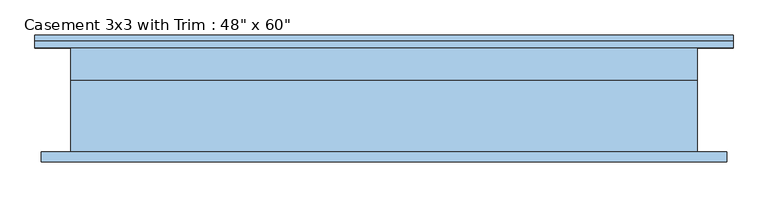
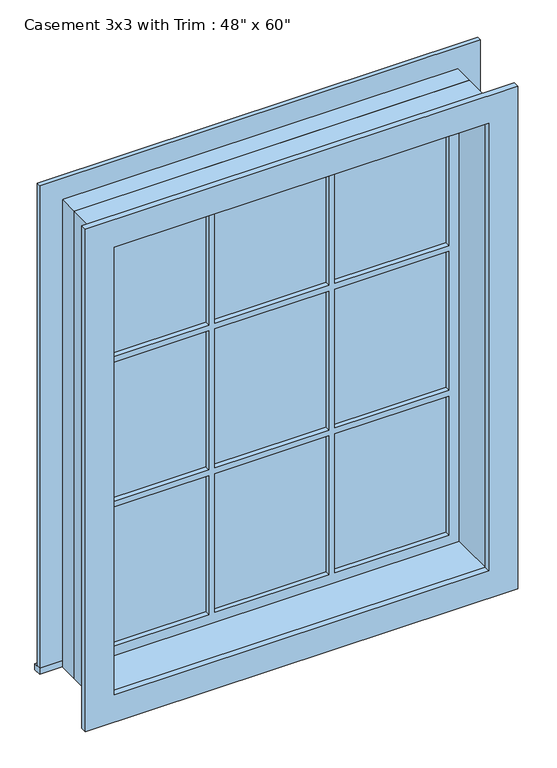
"""IFC4 building model written with IfcOpenShell, lengths in millimetres: window geometry."""

from ifc_helpers import new_model, si_unit, frame, origin, place, context, project, spatial, polyline, outline, extrude, source, transform, mapped, element, save


def window_26ecbd3e(model_context):
    return source(origin(), model_context, "Body", "SweptSolid", [
        extrude(outline(polyline([(-679.45, 127.0), (679.45, 127.0), (679.45, 101.6), (-679.45, 101.6), (-679.45, 127.0)])), frame((0.0, 0.0, 914.4), z_axis=(0.0, 0.0, 1.0), x_axis=(1.0, 0.0, 0.0)), (0.0, 0.0, 1.0), 19.05),
        extrude(outline(polyline([(2419.35, -590.55), (2419.35, 590.55), (933.45, 590.55), (933.45, 679.45), (2508.25, 679.45), (2508.25, -679.45), (933.45, -679.45), (933.45, -590.55), (2419.35, -590.55)])), frame((0.0, 101.6, 0.0), z_axis=(0.0, 1.0, 0.0), x_axis=(0.0, 0.0, 1.0)), (0.0, 0.0, 1.0), 12.7),
        extrude(outline(polyline([(194.7333333, 66.675), (546.1, 66.675), (546.1, 53.975), (194.7333333, 53.975), (194.7333333, 66.675)])), frame((0.0, 0.0, 1921.9333333), z_axis=(0.0, 0.0, 1.0), x_axis=(1.0, 0.0, 0.0)), (0.0, 0.0, 1.0), 452.9666667),
        extrude(outline(polyline([(-175.6833333, 66.675), (175.6833333, 66.675), (175.6833333, 53.975), (-175.6833333, 53.975), (-175.6833333, 66.675)])), frame((0.0, 0.0, 1921.9333333), z_axis=(0.0, 0.0, 1.0), x_axis=(1.0, 0.0, 0.0)), (0.0, 0.0, 1.0), 452.9666667),
        extrude(outline(polyline([(-546.1, 66.675), (-194.7333333, 66.675), (-194.7333333, 53.975), (-546.1, 53.975), (-546.1, 66.675)])), frame((0.0, 0.0, 1921.9333333), z_axis=(0.0, 0.0, 1.0), x_axis=(1.0, 0.0, 0.0)), (0.0, 0.0, 1.0), 452.9666667),
        extrude(outline(polyline([(-546.1, 66.675), (-194.7333333, 66.675), (-194.7333333, 53.975), (-546.1, 53.975), (-546.1, 66.675)])), frame((0.0, 0.0, 1449.9166667), z_axis=(0.0, 0.0, 1.0), x_axis=(1.0, 0.0, 0.0)), (0.0, 0.0, 1.0), 452.9666667),
        extrude(outline(polyline([(-175.6833333, 66.675), (175.6833333, 66.675), (175.6833333, 53.975), (-175.6833333, 53.975), (-175.6833333, 66.675)])), frame((0.0, 0.0, 1449.9166667), z_axis=(0.0, 0.0, 1.0), x_axis=(1.0, 0.0, 0.0)), (0.0, 0.0, 1.0), 452.9666667),
        extrude(outline(polyline([(194.7333333, 66.675), (546.1, 66.675), (546.1, 53.975), (194.7333333, 53.975), (194.7333333, 66.675)])), frame((0.0, 0.0, 1449.9166667), z_axis=(0.0, 0.0, 1.0), x_axis=(1.0, 0.0, 0.0)), (0.0, 0.0, 1.0), 452.9666667),
        extrude(outline(polyline([(194.7333333, 66.675), (546.1, 66.675), (546.1, 53.975), (194.7333333, 53.975), (194.7333333, 66.675)])), frame((0.0, 0.0, 977.9), z_axis=(0.0, 0.0, 1.0), x_axis=(1.0, 0.0, 0.0)), (0.0, 0.0, 1.0), 452.9666667),
        extrude(outline(polyline([(-175.6833333, 66.675), (175.6833333, 66.675), (175.6833333, 53.975), (-175.6833333, 53.975), (-175.6833333, 66.675)])), frame((0.0, 0.0, 977.9), z_axis=(0.0, 0.0, 1.0), x_axis=(1.0, 0.0, 0.0)), (0.0, 0.0, 1.0), 452.9666667),
        extrude(outline(polyline([(-546.1, 66.675), (-194.7333333, 66.675), (-194.7333333, 53.975), (-546.1, 53.975), (-546.1, 66.675)])), frame((0.0, 0.0, 977.9), z_axis=(0.0, 0.0, 1.0), x_axis=(1.0, 0.0, 0.0)), (0.0, 0.0, 1.0), 452.9666667),
        extrude(outline(polyline([(2495.55, 666.75), (2495.55, -666.75), (857.25, -666.75), (857.25, 666.75), (2495.55, 666.75)]), holes=[polyline([(2406.65, 577.85), (946.15, 577.85), (946.15, -577.85), (2406.65, -577.85), (2406.65, 577.85)])]), frame((0.0, -120.65, 0.0), z_axis=(0.0, 1.0, 0.0), x_axis=(0.0, 0.0, 1.0)), (0.0, 0.0, 1.0), 19.05),
        extrude(outline(polyline([(2419.35, -590.55), (933.45, -590.55), (933.45, 590.55), (2419.35, 590.55), (2419.35, -590.55)]), holes=[polyline([(2374.9, -194.7333333), (1921.9333333, -194.7333333), (1921.9333333, -546.1), (2374.9, -546.1), (2374.9, -194.7333333)]), polyline([(1902.8833333, -194.7333333), (1449.9166667, -194.7333333), (1449.9166667, -546.1), (1902.8833333, -546.1), (1902.8833333, -194.7333333)]), polyline([(1430.8666667, -194.7333333), (977.9, -194.7333333), (977.9, -546.1), (1430.8666667, -546.1), (1430.8666667, -194.7333333)]), polyline([(2374.9, 175.6833333), (1921.9333333, 175.6833333), (1921.9333333, -175.6833333), (2374.9, -175.6833333), (2374.9, 175.6833333)]), polyline([(1902.8833333, 175.6833333), (1449.9166667, 175.6833333), (1449.9166667, -175.6833333), (1902.8833333, -175.6833333), (1902.8833333, 175.6833333)]), polyline([(1430.8666667, 175.6833333), (977.9, 175.6833333), (977.9, -175.6833333), (1430.8666667, -175.6833333), (1430.8666667, 175.6833333)]), polyline([(2374.9, 546.1), (1921.9333333, 546.1), (1921.9333333, 194.7333333), (2374.9, 194.7333333), (2374.9, 546.1)]), polyline([(1902.8833333, 546.1), (1449.9166667, 546.1), (1449.9166667, 194.7333333), (1902.8833333, 194.7333333), (1902.8833333, 546.1)]), polyline([(1430.8666667, 546.1), (977.9, 546.1), (977.9, 194.7333333), (1430.8666667, 194.7333333), (1430.8666667, 546.1)])]), frame((0.0, 38.1, 0.0), z_axis=(0.0, 1.0, 0.0), x_axis=(0.0, 0.0, 1.0)), (0.0, 0.0, 1.0), 44.45),
        extrude(outline(polyline([(2438.4, -609.6), (914.4, -609.6), (914.4, 609.6), (2438.4, 609.6), (2438.4, -609.6)]), holes=[polyline([(2406.65, -577.85), (2406.65, 577.85), (946.15, 577.85), (946.15, -577.85), (2406.65, -577.85)])]), frame((0.0, -101.6, 0.0), z_axis=(0.0, 1.0, 0.0), x_axis=(0.0, 0.0, 1.0)), (0.0, 0.0, 1.0), 139.7),
        extrude(outline(polyline([(2438.4, 609.6), (2438.4, -609.6), (914.4, -609.6), (914.4, 609.6), (2438.4, 609.6)]), holes=[polyline([(2419.35, 590.55), (933.45, 590.55), (933.45, -590.55), (2419.35, -590.55), (2419.35, 590.55)])]), frame((0.0, 38.1, 0.0), z_axis=(0.0, 1.0, 0.0), x_axis=(0.0, 0.0, 1.0)), (0.0, 0.0, 1.0), 63.5),
    ])


if __name__ == "__main__":
    model = new_model("IFC4")
    model_context = context("Model", 3, world=origin())
    ifc_project = project(units=[si_unit("LENGTHUNIT", "METRE", prefix="MILLI")], contexts=[model_context])
    site = spatial("IfcSite", under=ifc_project)
    building = spatial("IfcBuilding", under=site)
    placement = place(None, origin())
    window_shape = window_26ecbd3e(model_context)
    element("IfcWindow", 1, ObjectType="Casement 3x3 with Trim : 48\" x 60\"", at=placement, inside=building, context=model_context, shape_type="MappedRepresentation", body=[
        mapped(window_shape, transform((0.0, 0.0, 0.0), x_axis=(1.0, 0.0, 0.0), y_axis=(0.0, 1.0, 0.0), z_axis=(0.0, 0.0, 1.0))),
    ])
    save(model, "model.ifc")

# Revit data of these elements
# Type "Casement 3x3 with Trim : 48\" x 60\""
#   Type Mark = "13"
#   Construction Type Id = "GSP4R"
#   Assembly Code = "B2020100"
#   Analytic Construction = "1/8 in Pilkington single glazing"
#   Visual Light Transmittance = 0.9
#   Solar Heat Gain Coefficient = 0.78
#   Heat Transfer Coefficient (U) = 0.6496 BTU/(h·ft²·°F)
#   Height = 5' - 0"
#   Default Sill Height = 3' - 0"
#   Trim Projection - Ext. = 0' - 0 1/2"
#   Trim Projection - Int. = 0' - 0 3/4"
#   Trim Width - Exterior = 0' - 3 1/2"
#   Trim Width - Interior = 0' - 3 1/2"
#   Width = 4' - 0"
#   Window Inset = 0' - 0 3/4"
#   Define Thermal Properties by = 1
#   Glass Pane Material = Glass
#   Sash Material = Sash
#   Trim Exterior Material = Trim
#   Trim Interior Material = Trim
#   Wall Closure = (empty or 0)
# Element 1 (IfcWindow, "Casement 3x3 with Trim : 48\" x 60\"")
#   Materials on its faces: "Sash", "Glass", "Trim"
# Materials
#   "Glass": class "Glass", colour RGB 0 128 192, transparency 0.75, Description = "Soda Lime Glass", Cost = 0
#   "Sash": class "Wood", colour RGB 224 178 126, transparency 0
#   "Trim": class "Wood", colour RGB 224 178 126, transparency 0
